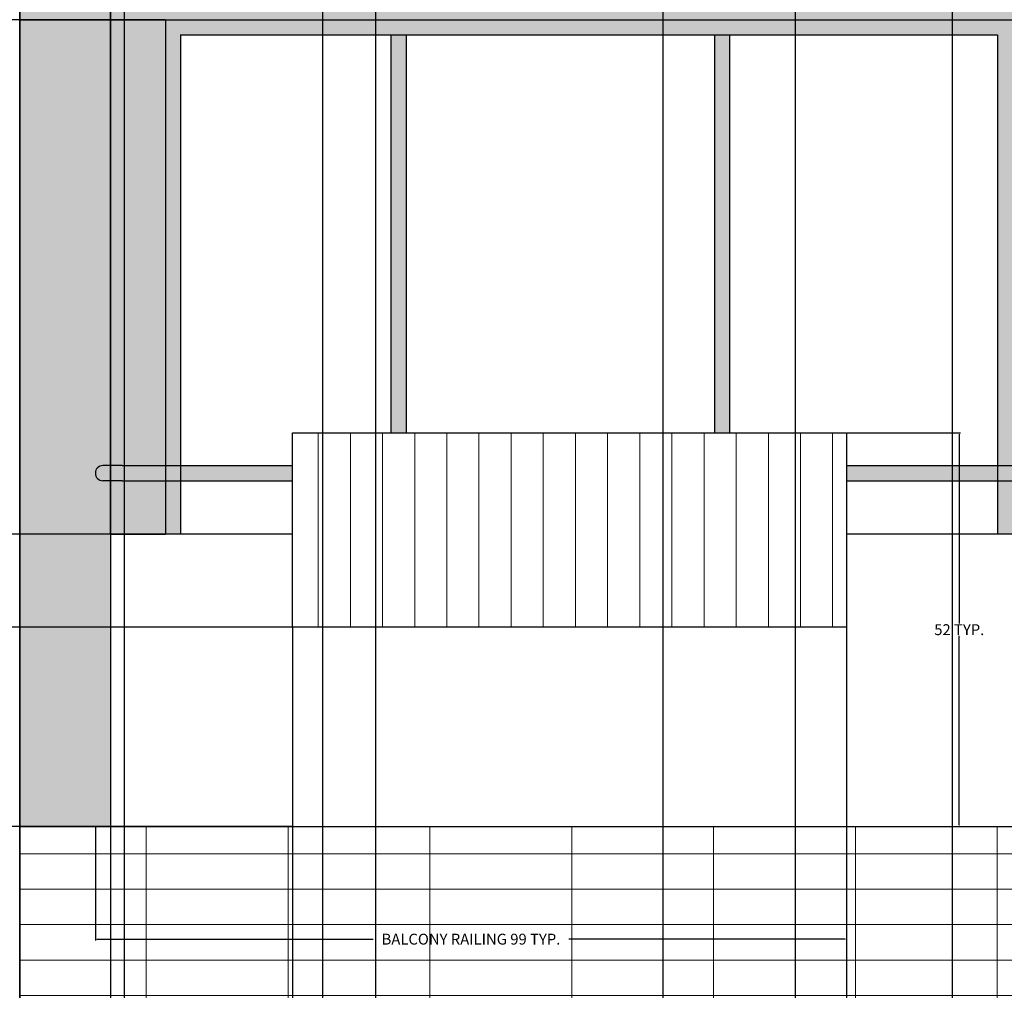
# Model space of a CAD drawing. Units: inches. Extents: x 241 to 943, y 109 to 1396.
# Tile 11 of 34: x 377 to 507, y 713 to 842. Entities that reach past the tile are written whole.
import ezdxf

# ---------------------------------------------------------------- set-up
doc = ezdxf.new("R2010")
doc.units = ezdxf.units.IN
doc.header["$MEASUREMENT"] = 0
for name, color, linetype, lineweight in [('A-ANNO-DIMS', 2, 'Continuous', 18), ('A-ELEV', 7, 'Continuous', 25), ('A-ELEV-SHAD', 9, 'Continuous', 13), ('A-GLAZ-PATT', 18, 'Continuous', 13), ('A-WALL-PATT', 8, 'Continuous', 13)]:
    doc.layers.add(name, color=color, linetype=linetype, lineweight=lineweight)
doc.styles.get("Standard").update_dxf_attribs({"font": 'arial.ttf'})
doc.dimstyles.get("Standard").update_dxf_attribs({"dimtxt": 1.4375, "dimasz": 0.18, "dimexe": 0.18, "dimexo": 0.0625, "dimgap": 0.09, "dimtad": 0, "dimtih": 1, "dimtoh": 1, "dimdec": 4, "dimzin": 0, "dimdsep": 46, "dimlunit": 4, "dimtxsty": 'Standard', "dimcen": 0.09, "dimadec": 0, "dimazin": 0, "dimtfac": 1, "dimtdec": 4, "dimtofl": 0, "dimtmove": 0, "dimatfit": 3, "dimfxl": 1, "dimtolj": 1, "dimtzin": 0, "dimarcsym": 0})

# ---------------------------------------------------------------- blocks, each defined once
blk = doc.blocks.new('BALCONY-RAIL')
for p, q in [((26.08, 26.37), (26.08, 52.06)), ((26.08, 52.06), (99.3, 52.06)), ((99.3, 52.06), (99.3, 26.37)), ((3.52, 47.73), (1, 47.73)), ((3.52, 47.73), (26.08, 47.73)), ((3.52, 45.73), (1, 45.73)), ((3.52, 45.73), (26.08, 45.73)), ((99.3, 26.37), (26.08, 26.37)), ((26.08, 26.37), (26.08, 0)), ((99.3, 26.37), (99.3, 0))]:
    blk.add_line(p, q)
blk.add_arc((1, 46.73), 1, 90, 270)
blk = doc.blocks.new('*D2')
at = {"layer": 'A-ANNO-DIMS', "color": 0, "lineweight": -2, "transparency": 16777216}
for p, q in [((387.04, 734.79), (387.04, 719.78)), ((486.34, 734.79), (486.34, 719.78)), ((387.22, 719.96), (423.76, 719.96)), ((486.16, 719.96), (449.62, 719.96))]:
    blk.add_line(p, q, dxfattribs=at)
at = {"layer": 'A-ANNO-DIMS', "color": 0, "transparency": 16777216}
for points in [[(387.22, 719.99), (387.22, 719.93), (387.04, 719.96)], [(486.16, 719.99), (486.16, 719.93), (486.34, 719.96)]]:
    blk.add_solid(points, dxfattribs=at)
at = {"layer": 'Defpoints', "color": 0, "transparency": 16777216}
for p in [(387.04, 734.85), (486.34, 734.85), (486.34, 719.96)]:
    blk.add_point(p, dxfattribs=at)
at = {"layer": 'A-ANNO-DIMS', "color": 0, "transparency": 16777216, "insert": (436.69, 719.96), "char_height": 1.4375, "attachment_point": 5}
blk.add_mtext('\\A1;BALCONY RAILING 99 TYP.', dxfattribs=at)
blk = doc.blocks.new('*D3')
at = {"layer": 'A-ANNO-DIMS', "color": 0, "lineweight": -2, "transparency": 16777216}
for p, q in [((486.4, 786.92), (501.42, 786.92)), ((501.24, 786.74), (501.24, 761.71)), ((501.24, 735.03), (501.24, 760.06)), ((486.4, 734.85), (501.42, 734.85))]:
    blk.add_line(p, q, dxfattribs=at)
at = {"layer": 'A-ANNO-DIMS', "color": 0, "transparency": 16777216}
for points in [[(501.21, 786.74), (501.27, 786.74), (501.24, 786.92)], [(501.21, 735.03), (501.27, 735.03), (501.24, 734.85)]]:
    blk.add_solid(points, dxfattribs=at)
at = {"layer": 'Defpoints', "color": 0, "transparency": 16777216}
for p in [(486.34, 786.92), (501.24, 786.92), (486.34, 734.85)]:
    blk.add_point(p, dxfattribs=at)
at = {"layer": 'A-ANNO-DIMS', "color": 0, "transparency": 16777216, "insert": (501.24, 760.88), "char_height": 1.4375, "attachment_point": 5}
blk.add_mtext('\\A1;52 TYP.', dxfattribs=at)
blk = doc.blocks.new('*D7')
at = {"layer": 'A-ANNO-DIMS', "color": 0, "lineweight": -2, "transparency": 16777216}
for p, q in [((508.24, 1336.12), (244.31, 1336.12)), ((244.49, 1335.94), (244.49, 753.25)), ((244.49, 168.92), (244.49, 751.6)), ((303.17, 168.74), (244.31, 168.74))]:
    blk.add_line(p, q, dxfattribs=at)
at = {"layer": 'A-ANNO-DIMS', "color": 0, "transparency": 16777216}
for points in [[(244.46, 1335.94), (244.52, 1335.94), (244.49, 1336.12)], [(244.46, 168.92), (244.52, 168.92), (244.49, 168.74)]]:
    blk.add_solid(points, dxfattribs=at)
at = {"layer": 'Defpoints', "color": 0, "transparency": 16777216}
for p in [(244.49, 1336.12), (508.31, 1336.12), (303.24, 168.74)]:
    blk.add_point(p, dxfattribs=at)
at = {"layer": 'A-ANNO-DIMS', "color": 0, "transparency": 16777216, "insert": (244.49, 752.43), "char_height": 1.438, "attachment_point": 5}
blk.add_mtext('\\A1;1167.4', dxfattribs=at)
blk = doc.blocks.new('*D8')
at = {"layer": 'A-ANNO-DIMS', "color": 0, "lineweight": -2, "transparency": 16777216}
for p, q in [((377.04, 396.94), (377.04, 1395.05)), ((377.22, 1394.87), (380.96, 1394.87)), ((390.71, 1394.87), (386.97, 1394.87)), ((390.89, 384.24), (390.89, 1395.05))]:
    blk.add_line(p, q, dxfattribs=at)
at = {"layer": 'A-ANNO-DIMS', "color": 0, "transparency": 16777216}
for points in [[(377.22, 1394.9), (377.22, 1394.84), (377.04, 1394.87)], [(390.71, 1394.9), (390.71, 1394.84), (390.89, 1394.87)]]:
    blk.add_solid(points, dxfattribs=at)
at = {"layer": 'Defpoints', "color": 0, "transparency": 16777216}
for p in [(390.89, 1394.87), (377.04, 396.88), (390.89, 384.18)]:
    blk.add_point(p, dxfattribs=at)
at = {"layer": 'A-ANNO-DIMS', "color": 0, "transparency": 16777216, "insert": (383.97, 1394.87), "char_height": 1.438, "attachment_point": 5}
blk.add_mtext('\\A1;13.856', dxfattribs=at)
blk = doc.blocks.new('*D9')
at = {"layer": 'A-ANNO-DIMS', "color": 0, "lineweight": -2, "transparency": 16777216}
for p, q in [((390.89, 384.24), (390.89, 1395.05)), ((391.07, 1394.87), (424.13, 1394.87)), ((461.93, 1394.87), (428.87, 1394.87)), ((462.11, 384.24), (462.11, 1395.05))]:
    blk.add_line(p, q, dxfattribs=at)
at = {"layer": 'A-ANNO-DIMS', "color": 0, "transparency": 16777216}
for points in [[(391.07, 1394.9), (391.07, 1394.84), (390.89, 1394.87)], [(461.93, 1394.9), (461.93, 1394.84), (462.11, 1394.87)]]:
    blk.add_solid(points, dxfattribs=at)
at = {"layer": 'Defpoints', "color": 0, "transparency": 16777216}
for p in [(462.11, 1394.87), (390.89, 384.18), (462.11, 384.18)]:
    blk.add_point(p, dxfattribs=at)
at = {"layer": 'A-ANNO-DIMS', "color": 0, "transparency": 16777216, "insert": (426.5, 1394.87), "char_height": 1.438, "attachment_point": 5}
blk.add_mtext('\\A1;71.21', dxfattribs=at)
blk = doc.blocks.new('*D10')
at = {"layer": 'A-ANNO-DIMS', "color": 0, "lineweight": -2, "transparency": 16777216}
for p, q in [((462.11, 384.24), (462.11, 1395.05)), ((462.29, 1394.87), (468.4, 1394.87)), ((479.42, 1394.87), (473.3, 1394.87)), ((479.6, 384.24), (479.6, 1395.05))]:
    blk.add_line(p, q, dxfattribs=at)
at = {"layer": 'A-ANNO-DIMS', "color": 0, "transparency": 16777216}
for points in [[(462.29, 1394.9), (462.29, 1394.84), (462.11, 1394.87)], [(479.42, 1394.9), (479.42, 1394.84), (479.6, 1394.87)]]:
    blk.add_solid(points, dxfattribs=at)
at = {"layer": 'Defpoints', "color": 0, "transparency": 16777216}
for p in [(479.6, 1394.87), (462.11, 384.18), (479.6, 384.18)]:
    blk.add_point(p, dxfattribs=at)
at = {"layer": 'A-ANNO-DIMS', "color": 0, "transparency": 16777216, "insert": (470.85, 1394.87), "char_height": 1.438, "attachment_point": 5}
blk.add_mtext('\\A1;17.49', dxfattribs=at)
blk = doc.blocks.new('*D11')
at = {"layer": 'A-ANNO-DIMS', "color": 0, "lineweight": -2, "transparency": 16777216}
for p, q in [((500.33, 384.24), (500.33, 1395.05)), ((500.51, 1394.87), (513.31, 1394.87)), ((530.05, 1394.87), (517.25, 1394.87)), ((530.23, 384.24), (530.23, 1395.05))]:
    blk.add_line(p, q, dxfattribs=at)
at = {"layer": 'A-ANNO-DIMS', "color": 0, "transparency": 16777216}
for points in [[(500.51, 1394.9), (500.51, 1394.84), (500.33, 1394.87)], [(530.05, 1394.9), (530.05, 1394.84), (530.23, 1394.87)]]:
    blk.add_solid(points, dxfattribs=at)
at = {"layer": 'Defpoints', "color": 0, "transparency": 16777216}
for p in [(530.23, 1394.87), (500.33, 384.18), (530.23, 384.18)]:
    blk.add_point(p, dxfattribs=at)
at = {"layer": 'A-ANNO-DIMS', "color": 0, "transparency": 16777216, "insert": (515.28, 1394.87), "char_height": 1.438, "attachment_point": 5}
blk.add_mtext('\\A1;29.9', dxfattribs=at)
blk = doc.blocks.new('*D35')
at = {"layer": 'A-ANNO-DIMS', "color": 0, "lineweight": -2, "transparency": 16777216}
for p, q in [((388.98, 773.49), (244.31, 773.49)), ((244.49, 773.31), (244.49, 755)), ((244.49, 735.03), (244.49, 753.35)), ((388.98, 734.85), (244.31, 734.85))]:
    blk.add_line(p, q, dxfattribs=at)
at = {"layer": 'A-ANNO-DIMS', "color": 0, "transparency": 16777216}
for points in [[(244.46, 773.31), (244.52, 773.31), (244.49, 773.49)], [(244.46, 735.03), (244.52, 735.03), (244.49, 734.85)]]:
    blk.add_solid(points, dxfattribs=at)
at = {"layer": 'Defpoints', "color": 0, "transparency": 16777216}
for p in [(244.49, 773.49), (389.04, 773.49), (389.04, 734.85)]:
    blk.add_point(p, dxfattribs=at)
at = {"layer": 'A-ANNO-DIMS', "color": 0, "transparency": 16777216, "insert": (244.49, 754.17), "char_height": 1.438, "attachment_point": 5}
blk.add_mtext('\\A1;38.64', dxfattribs=at)
blk = doc.blocks.new('*D36')
at = {"layer": 'A-ANNO-DIMS', "color": 0, "lineweight": -2, "transparency": 16777216}
for p, q in [((396.25, 841.54), (244.31, 841.54)), ((244.49, 841.36), (244.49, 808.34)), ((244.49, 773.67), (244.49, 806.69)), ((396.25, 773.49), (244.31, 773.49))]:
    blk.add_line(p, q, dxfattribs=at)
at = {"layer": 'A-ANNO-DIMS', "color": 0, "transparency": 16777216}
for points in [[(244.46, 841.36), (244.52, 841.36), (244.49, 841.54)], [(244.46, 773.67), (244.52, 773.67), (244.49, 773.49)]]:
    blk.add_solid(points, dxfattribs=at)
at = {"layer": 'Defpoints', "color": 0, "transparency": 16777216}
for p in [(244.49, 841.54), (396.31, 841.54), (396.31, 773.49)]:
    blk.add_point(p, dxfattribs=at)
at = {"layer": 'A-ANNO-DIMS', "color": 0, "transparency": 16777216, "insert": (244.49, 807.51), "char_height": 1.438, "attachment_point": 5}
blk.add_mtext('\\A1;68.05', dxfattribs=at)
blk = doc.blocks.new('*D61')
at = {"layer": 'A-ANNO-DIMS', "color": 0, "lineweight": -2, "transparency": 16777216}
for p, q in [((377.04, 400.89), (377.04, 1395.05)), ((377.22, 1394.87), (398.03, 1394.87)), ((423.93, 1394.87), (403.12, 1394.87)), ((424.11, 568.89), (424.11, 1395.05))]:
    blk.add_line(p, q, dxfattribs=at)
at = {"layer": 'A-ANNO-DIMS', "color": 0, "transparency": 16777216}
for points in [[(377.22, 1394.9), (377.22, 1394.84), (377.04, 1394.87)], [(423.93, 1394.9), (423.93, 1394.84), (424.11, 1394.87)]]:
    blk.add_solid(points, dxfattribs=at)
at = {"layer": 'Defpoints', "color": 0, "transparency": 16777216}
for p in [(424.11, 1394.87), (424.11, 568.83), (377.04, 400.83)]:
    blk.add_point(p, dxfattribs=at)
at = {"layer": 'A-ANNO-DIMS', "color": 0, "transparency": 16777216, "insert": (400.57, 1394.87), "char_height": 1.438, "attachment_point": 5}
blk.add_mtext('\\A1;47.07', dxfattribs=at)
blk = doc.blocks.new('*D62')
at = {"layer": 'A-ANNO-DIMS', "color": 0, "lineweight": -2, "transparency": 16777216}
for p, q in [((424.11, 568.89), (424.11, 1395.05)), ((424.29, 1394.87), (492.35, 1394.87)), ((565.02, 1394.87), (496.96, 1394.87)), ((565.2, 568.89), (565.2, 1395.05))]:
    blk.add_line(p, q, dxfattribs=at)
at = {"layer": 'A-ANNO-DIMS', "color": 0, "transparency": 16777216}
for points in [[(424.29, 1394.9), (424.29, 1394.84), (424.11, 1394.87)], [(565.02, 1394.9), (565.02, 1394.84), (565.2, 1394.87)]]:
    blk.add_solid(points, dxfattribs=at)
at = {"layer": 'Defpoints', "color": 0, "transparency": 16777216}
for p in [(565.2, 1394.87), (424.11, 568.83), (565.2, 568.83)]:
    blk.add_point(p, dxfattribs=at)
at = {"layer": 'A-ANNO-DIMS', "color": 0, "transparency": 16777216, "insert": (494.66, 1394.87), "char_height": 1.438, "attachment_point": 5}
blk.add_mtext('\\A1;141.1', dxfattribs=at)
blk = doc.blocks.new('*D65')
at = {"layer": 'A-ANNO-DIMS', "color": 0, "lineweight": -2, "transparency": 16777216}
for p, q in [((424.11, 700.85), (424.11, 1395.05)), ((424.29, 1394.87), (505.52, 1394.87)), ((592.77, 1394.87), (511.54, 1394.87)), ((592.95, 700.85), (592.95, 1395.05))]:
    blk.add_line(p, q, dxfattribs=at)
at = {"layer": 'A-ANNO-DIMS', "color": 0, "transparency": 16777216}
for points in [[(424.29, 1394.9), (424.29, 1394.84), (424.11, 1394.87)], [(592.77, 1394.9), (592.77, 1394.84), (592.95, 1394.87)]]:
    blk.add_solid(points, dxfattribs=at)
at = {"layer": 'Defpoints', "color": 0, "transparency": 16777216}
for p in [(592.95, 1394.87), (424.11, 700.79), (592.95, 700.79)]:
    blk.add_point(p, dxfattribs=at)
at = {"layer": 'A-ANNO-DIMS', "color": 0, "transparency": 16777216, "insert": (508.53, 1394.87), "char_height": 1.438, "attachment_point": 5}
blk.add_mtext('\\A1;168.85', dxfattribs=at)
blk = doc.blocks.new('*D67')
at = {"layer": 'A-ANNO-DIMS', "color": 0, "lineweight": -2, "transparency": 16777216}
for p, q in [((389.04, 773.55), (389.04, 1395.05)), ((389.22, 1394.87), (495.34, 1394.87)), ((607.64, 1394.87), (501.52, 1394.87)), ((607.82, 773.55), (607.82, 1395.05))]:
    blk.add_line(p, q, dxfattribs=at)
at = {"layer": 'A-ANNO-DIMS', "color": 0, "transparency": 16777216}
for points in [[(389.22, 1394.9), (389.22, 1394.84), (389.04, 1394.87)], [(607.64, 1394.9), (607.64, 1394.84), (607.82, 1394.87)]]:
    blk.add_solid(points, dxfattribs=at)
at = {"layer": 'Defpoints', "color": 0, "transparency": 16777216}
for p in [(607.82, 1394.87), (389.04, 773.49), (607.82, 773.49)]:
    blk.add_point(p, dxfattribs=at)
at = {"layer": 'A-ANNO-DIMS', "color": 0, "transparency": 16777216, "insert": (498.43, 1394.87), "char_height": 1.438, "attachment_point": 5}
blk.add_mtext('\\A1;218.77', dxfattribs=at)
blk = doc.blocks.new('*D79')
at = {"layer": 'A-ANNO-DIMS', "color": 0, "lineweight": -2, "transparency": 16777216}
for p, q in [((479.6, 384.24), (479.6, 1395.05)), ((479.78, 1394.87), (486.88, 1394.87)), ((500.15, 1394.87), (493.05, 1394.87)), ((500.33, 384.24), (500.33, 1395.05))]:
    blk.add_line(p, q, dxfattribs=at)
at = {"layer": 'A-ANNO-DIMS', "color": 0, "transparency": 16777216}
for points in [[(479.78, 1394.9), (479.78, 1394.84), (479.6, 1394.87)], [(500.15, 1394.9), (500.15, 1394.84), (500.33, 1394.87)]]:
    blk.add_solid(points, dxfattribs=at)
at = {"layer": 'Defpoints', "color": 0, "transparency": 16777216}
for p in [(500.33, 1394.87), (479.6, 384.18), (500.33, 384.18)]:
    blk.add_point(p, dxfattribs=at)
at = {"layer": 'A-ANNO-DIMS', "color": 0, "transparency": 16777216, "insert": (489.96, 1394.87), "char_height": 1.438, "attachment_point": 5}
blk.add_mtext('\\A1;20.736', dxfattribs=at)
blk = doc.blocks.new('*D91')
at = {"layer": 'A-ANNO-DIMS', "color": 0, "lineweight": -2, "transparency": 16777216}
for p, q in [((377.04, 1070.79), (377.04, 109.81)), ((389.04, 1070.79), (389.04, 109.81)), ((377.22, 109.99), (380.04, 109.99)), ((388.86, 109.99), (386.04, 109.99))]:
    blk.add_line(p, q, dxfattribs=at)
at = {"layer": 'A-ANNO-DIMS', "color": 0, "transparency": 16777216}
for points in [[(377.22, 110.02), (377.22, 109.96), (377.04, 109.99)], [(388.86, 110.02), (388.86, 109.96), (389.04, 109.99)]]:
    blk.add_solid(points, dxfattribs=at)
at = {"layer": 'Defpoints', "color": 0, "transparency": 16777216}
for p in [(377.04, 1070.85), (389.04, 1070.85), (389.04, 109.99)]:
    blk.add_point(p, dxfattribs=at)
at = {"layer": 'A-ANNO-DIMS', "color": 0, "transparency": 16777216, "insert": (383.04, 109.99), "char_height": 1.438, "attachment_point": 5}
blk.add_mtext('\\A1;12.004', dxfattribs=at)
blk = doc.blocks.new('*D99')
at = {"layer": 'A-ANNO-DIMS', "color": 0, "lineweight": -2, "transparency": 16777216}
for p, q in [((417.09, 181.71), (417.09, 1395.05)), ((417.27, 1394.87), (539.16, 1394.87)), ((667.21, 1394.87), (545.33, 1394.87)), ((667.39, 214.58), (667.39, 1395.05))]:
    blk.add_line(p, q, dxfattribs=at)
at = {"layer": 'A-ANNO-DIMS', "color": 0, "transparency": 16777216}
for points in [[(417.27, 1394.9), (417.27, 1394.84), (417.09, 1394.87)], [(667.21, 1394.9), (667.21, 1394.84), (667.39, 1394.87)]]:
    blk.add_solid(points, dxfattribs=at)
at = {"layer": 'Defpoints', "color": 0, "transparency": 16777216}
for p in [(667.39, 1394.87), (667.39, 214.52), (417.09, 181.65)]:
    blk.add_point(p, dxfattribs=at)
at = {"layer": 'A-ANNO-DIMS', "color": 0, "transparency": 16777216, "insert": (542.24, 1394.87), "char_height": 1.438, "attachment_point": 5}
blk.add_mtext('\\A1;250.30', dxfattribs=at)
blk = doc.blocks.new('*D147')
at = {"layer": 'A-ANNO-DIMS', "color": 0, "lineweight": -2, "transparency": 16777216}
for p, q in [((389.04, 734.79), (389.04, 109.81)), ((413.12, 734.79), (413.12, 109.81)), ((389.22, 109.99), (398, 109.99)), ((412.94, 109.99), (404.17, 109.99))]:
    blk.add_line(p, q, dxfattribs=at)
at = {"layer": 'A-ANNO-DIMS', "color": 0, "transparency": 16777216}
for points in [[(389.22, 110.02), (389.22, 109.96), (389.04, 109.99)], [(412.94, 110.02), (412.94, 109.96), (413.12, 109.99)]]:
    blk.add_solid(points, dxfattribs=at)
at = {"layer": 'Defpoints', "color": 0, "transparency": 16777216}
for p in [(389.04, 734.85), (413.12, 734.85), (413.12, 109.99)]:
    blk.add_point(p, dxfattribs=at)
at = {"layer": 'A-ANNO-DIMS', "color": 0, "transparency": 16777216, "insert": (401.08, 109.99), "char_height": 1.438, "attachment_point": 5}
blk.add_mtext('\\A1;24.076', dxfattribs=at)
blk = doc.blocks.new('*D148')
at = {"layer": 'A-ANNO-DIMS', "color": 0, "lineweight": -2, "transparency": 16777216}
for p, q in [((413.12, 734.79), (413.12, 109.81)), ((486.34, 734.79), (486.34, 109.81)), ((413.3, 109.99), (447.23, 109.99)), ((486.16, 109.99), (452.23, 109.99))]:
    blk.add_line(p, q, dxfattribs=at)
at = {"layer": 'A-ANNO-DIMS', "color": 0, "transparency": 16777216}
for points in [[(413.3, 110.02), (413.3, 109.96), (413.12, 109.99)], [(486.16, 110.02), (486.16, 109.96), (486.34, 109.99)]]:
    blk.add_solid(points, dxfattribs=at)
at = {"layer": 'Defpoints', "color": 0, "transparency": 16777216}
for p in [(413.12, 734.85), (486.34, 734.85), (486.34, 109.99)]:
    blk.add_point(p, dxfattribs=at)
at = {"layer": 'A-ANNO-DIMS', "color": 0, "transparency": 16777216, "insert": (449.73, 109.99), "char_height": 1.438, "attachment_point": 5}
blk.add_mtext('\\A1;73.22', dxfattribs=at)
blk = doc.blocks.new('*D149')
at = {"layer": 'A-ANNO-DIMS', "color": 0, "lineweight": -2, "transparency": 16777216}
for p, q in [((413.06, 761.23), (244.31, 761.23)), ((244.49, 761.05), (244.49, 748.87)), ((244.49, 735.03), (244.49, 747.22)), ((413.06, 734.85), (244.31, 734.85))]:
    blk.add_line(p, q, dxfattribs=at)
at = {"layer": 'A-ANNO-DIMS', "color": 0, "transparency": 16777216}
for points in [[(244.46, 761.05), (244.52, 761.05), (244.49, 761.23)], [(244.46, 735.03), (244.52, 735.03), (244.49, 734.85)]]:
    blk.add_solid(points, dxfattribs=at)
at = {"layer": 'Defpoints', "color": 0, "transparency": 16777216}
for p in [(244.49, 761.23), (413.12, 761.23), (413.12, 734.85)]:
    blk.add_point(p, dxfattribs=at)
at = {"layer": 'A-ANNO-DIMS', "color": 0, "transparency": 16777216, "insert": (244.49, 748.04), "char_height": 1.438, "attachment_point": 5}
blk.add_mtext('\\A1;26.375', dxfattribs=at)

msp = doc.modelspace()

# ---------------------------------------------------------------- hatches: boundary and pattern name
at = {"layer": 'A-ELEV-SHAD'}
h = msp.add_hatch(color=256, dxfattribs=at)
h.dxf.hatch_style = 1
h.paths.add_polyline_path([(508.3064, 1070.8538), (377.0391, 1070.8538), (377.0391, 1009.5382), (508.3064, 1009.5382)])
h.paths.add_polyline_path([(508.3064, 1238.8538), (377.0391, 1238.8538), (377.0391, 1177.5382), (508.3064, 1177.5382)])
h.paths.add_polyline_path([(581.3632, 902.8538), (568.1348, 902.8538), (553.5166, 902.8538), (377.0391, 902.8538), (377.0391, 841.5382), (553.5166, 841.5382), (564.8076, 841.5382), (581.3632, 841.5382)])
h.paths.add_polyline_path([(820.8374, 1275.9142), (747.7579, 1275.9142), (747.7579, 1238.8538), (820.8374, 1238.8538)])
h.paths.add_polyline_path([(820.8374, 1238.8538), (747.7579, 1238.8538), (747.9341, 1223.0633), (820.8374, 1223.0633)])
h.paths.add_polyline_path([(396.3125, 841.5382), (377.0391, 841.5382), (377.0391, 734.8538), (389.0429, 734.8538), (389.0429, 735.188), (389.0429, 773.4916), (396.3125, 773.4916), (396.3125, 780.5808), (390.5597, 780.5808), (388.0428, 780.5808, -1), (388.0428, 782.5808), (390.5597, 782.5808), (396.3125, 782.5808)])
h = msp.add_hatch(color=256, dxfattribs=at)
h.dxf.hatch_style = 1
h.paths.add_polyline_path([(537.4269, 698.7912), (534.1778, 698.7912), (534.1778, 659.3434), (537.4269, 659.3434)])
h.paths.add_polyline_path([(508.0803, 698.7912), (450.9259, 698.7912), (450.9259, 659.3434), (452.9259, 659.3434), (452.9259, 696.7912), (506.0803, 696.7912), (506.0803, 659.3434), (508.0803, 659.3434)])
h.paths.add_polyline_path([(481.5031, 696.7912), (479.5031, 696.7912), (479.5031, 659.3434), (481.5031, 659.3434)], flags=17)
h.paths.add_polyline_path([(481.5031, 657.3434), (479.5031, 657.3434), (479.5031, 653.3371), (481.5031, 653.3371)], flags=17)
h.paths.add_polyline_path([(508.0803, 657.3434), (506.0803, 657.3434), (506.0803, 653.3371), (452.9259, 653.3371), (452.9259, 657.3434), (450.9259, 657.3434), (450.9259, 651.3371), (508.0803, 651.3371)])
h.paths.add_polyline_path([(428.1173, 839.5382), (426.1173, 839.5382), (426.1173, 786.9154), (428.1173, 786.9154)], flags=17)
h.paths.add_polyline_path([(470.8692, 839.5382), (468.8692, 839.5382), (468.8692, 786.9154), (470.8692, 786.9154)], flags=17)
h.paths.add_polyline_path([(508.3064, 841.5382), (396.3125, 841.5382), (396.3125, 782.5808), (398.3125, 782.5808), (398.3125, 839.5382), (506.3064, 839.5382), (506.3064, 782.5808), (508.3064, 782.5808)])
h.paths.add_polyline_path([(398.3125, 780.5808), (396.3125, 780.5808), (396.3125, 773.4916), (398.3125, 773.4916)])
h.paths.add_polyline_path([(508.3064, 780.5808), (506.3064, 780.5808), (506.3064, 773.4916), (508.3064, 773.4916)])
h.paths.add_polyline_path([(715.6236, 841.5382), (678.2674, 841.5382), (678.2674, 734.8538), (715.6236, 734.8538)])
h.paths.add_polyline_path([(680.2674, 839.5382), (682.4526, 839.5382), (713.6236, 839.5382), (713.6236, 736.9235), (690.2047, 736.9235), (680.2674, 736.9235)], flags=16)
h.paths.add_polyline_path([(792.691, 841.5382), (747.7579, 841.5382), (747.7579, 734.8538), (754.5373, 734.8538), (754.5373, 736.9235), (754.5373, 839.5382), (756.7224, 839.5382), (787.8934, 839.5382), (787.8934, 765.9585), (792.691, 765.9585)])
h.paths.add_polyline_path([(659.2925, 1009.5382), (657.2925, 1009.5382), (657.2925, 902.8538), (659.2925, 902.8538)])
h.paths.add_polyline_path([(751.5078, 976.6275), (712.5839, 976.6275), (712.5839, 974.6275), (751.5078, 974.6275)])
h.paths.add_polyline_path([(470.8692, 1007.5382), (468.8692, 1007.5382), (468.8692, 954.9154), (470.8692, 954.9154)], flags=17)
h.paths.add_polyline_path([(508.3064, 1009.5382), (396.3125, 1009.5382), (396.3125, 950.5808), (398.3125, 950.5808), (398.3125, 1007.5382), (506.3064, 1007.5382), (506.3064, 950.5808), (508.3064, 950.5808)])
h.paths.add_polyline_path([(428.1173, 1007.5382), (426.1173, 1007.5382), (426.1173, 954.9154), (428.1173, 954.9154)], flags=17)
h.paths.add_polyline_path([(398.3125, 948.5808), (396.3125, 948.5808), (396.3125, 941.4916), (398.3125, 941.4916)])
h.paths.add_polyline_path([(508.3064, 948.5808), (506.3064, 948.5808), (506.3064, 941.4916), (508.3064, 941.4916)])
h.paths.add_polyline_path([(428.1173, 1175.5382), (426.1173, 1175.5382), (426.1173, 1122.9154), (428.1173, 1122.9154)], flags=17)
h.paths.add_polyline_path([(508.3064, 1177.5382), (396.3125, 1177.5382), (396.3125, 1118.5808), (398.3125, 1118.5808), (398.3125, 1175.5382), (506.3064, 1175.5382), (506.3064, 1118.5808), (506.8039, 1118.5808, -1), (506.8039, 1116.5808), (506.3064, 1116.5808), (506.3064, 1109.4916), (508.3064, 1109.4916)])
h.paths.add_polyline_path([(470.8692, 1175.5382), (468.8692, 1175.5382), (468.8692, 1122.9154), (470.8692, 1122.9154)], flags=17)
h.paths.add_polyline_path([(398.3125, 1116.5808), (396.3125, 1116.5808), (396.3125, 1109.4916), (398.3125, 1109.4916)], flags=17)
h.paths.add_polyline_path([(724.819, 1177.7336), (533.952, 1177.7336), (533.952, 1108.1686), (724.819, 1108.1686)])
h.paths.add_polyline_path([(535.952, 1175.7336), (722.819, 1175.7336), (722.819, 1110.1686), (535.952, 1110.1686)], flags=0)
h.paths.add_polyline_path([(622.521, 1136.0739), (643.4534, 1136.0739), (643.4534, 1134.0739), (622.521, 1134.0739)], flags=0)
h.paths.add_polyline_path([(722.819, 1175.7336), (535.952, 1175.7336), (535.952, 1110.1686), (722.819, 1110.1686)], flags=16)
h.paths.add_polyline_path([(565.947, 1151.5772), (535.952, 1151.5772), (535.952, 1149.5772), (565.947, 1149.5772)], flags=0)
at = {"layer": 'A-GLAZ-PATT'}
h = msp.add_hatch(dxfattribs=at)
h.set_pattern_fill('ANSI31', color=256, scale=34, angle=45)
h.paths.add_polyline_path([(486.3418, 786.9154), (413.1187, 786.9154), (413.1187, 761.2284), (486.3418, 761.2284)])
h.paths.add_polyline_path([(486.3418, 954.9154), (413.1187, 954.9154), (413.1187, 929.2284), (486.3418, 929.2284)])
h.paths.add_polyline_path([(462.1074, 289.6933), (390.895, 289.6933), (390.895, 277.4626), (390.895, 274.3507), (462.1074, 274.3507), (462.1074, 277.4626)])
h.paths.add_polyline_path([(500.3323, 289.6933), (479.596, 289.6933), (479.596, 274.3507), (500.3323, 274.3507)])
h.paths.add_polyline_path([(450.9259, 566.8295), (426.1086, 566.8295), (426.1086, 498.4395), (446.4348, 498.4395), (446.4348, 519.3754), (450.9259, 519.3754), (450.9259, 525.3816), (445.5808, 525.3816, -1), (445.5808, 527.3816), (450.9259, 527.3816)])
h.paths.add_polyline_path([(563.2023, 508.9074), (534.1778, 508.9074), (508.1906, 508.9074), (508.1906, 498.4395), (563.2023, 498.4395)])
h.paths.add_polyline_path([(747.6328, 700.7912), (712.0171, 700.7912), (712.0171, 628.4013), (747.6328, 628.4013)])
h.paths.add_polyline_path([(446.4348, 643.7483), (426.1086, 643.7483), (426.1086, 630.4013), (446.4348, 630.4013)])
h.paths.add_polyline_path([(564.8076, 841.5382), (553.5166, 841.5382), (508.3064, 841.5382), (508.3064, 782.5808), (564.8076, 782.5808)])
h.paths.add_polyline_path([(564.8076, 780.5808), (508.3064, 780.5808), (508.3064, 773.4916), (564.8076, 773.4916)])
h.paths.add_polyline_path([(792.691, 762.5799), (759.6248, 762.5799), (759.6248, 736.9235), (759.6248, 734.8538), (792.691, 734.8538)])
h.paths.add_polyline_path([(564.8076, 1009.5382), (553.5166, 1009.5382), (508.3064, 1009.5382), (508.3064, 950.5808), (562.3033, 950.5808, -1), (562.3033, 948.5808), (508.3064, 948.5808), (508.3064, 941.4916), (564.8076, 941.4916)])
h.paths.add_polyline_path([(486.3418, 1122.9154), (413.1187, 1122.9154), (413.1187, 1097.2284), (486.3418, 1097.2284)])
h = msp.add_hatch(color=256, dxfattribs=at)
h.dxf.hatch_style = 1
h.paths.add_polyline_path([(396.3125, 1118.5808), (390.5597, 1118.5808), (388.0428, 1118.5808, 1), (388.0428, 1116.5808), (390.5597, 1116.5808), (396.3125, 1116.5808)])
h.paths.add_polyline_path([(398.3125, 1118.5808), (396.3125, 1118.5808), (396.3125, 1116.5808), (398.3125, 1116.5808)])
h.paths.add_polyline_path([(413.1187, 1118.5808), (398.3125, 1118.5808), (398.3125, 1116.5808), (413.1187, 1116.5808)])
h.paths.add_polyline_path([(506.3064, 1118.5808), (486.3418, 1118.5808), (486.3418, 1116.5808), (506.3064, 1116.5808)])
h.paths.add_polyline_path([(506.8039, 1118.5808), (506.3064, 1118.5808), (506.3064, 1116.5808), (506.8039, 1116.5808, 1)])
h.paths.add_polyline_path([(396.3125, 950.5808), (390.5597, 950.5808), (388.0428, 950.5808, 1), (388.0428, 948.5808), (390.5597, 948.5808), (396.3125, 948.5808)])
h.paths.add_polyline_path([(398.3125, 950.5808), (396.3125, 950.5808), (396.3125, 948.5808), (398.3125, 948.5808)])
h.paths.add_polyline_path([(413.1187, 950.5808), (398.3125, 950.5808), (398.3125, 948.5808), (413.1187, 948.5808)])
h.paths.add_polyline_path([(506.3064, 950.5808), (486.3418, 950.5808), (486.3418, 948.5808), (506.3064, 948.5808)])
h.paths.add_polyline_path([(508.3064, 950.5808), (506.3064, 950.5808), (506.3064, 948.5808), (508.3064, 948.5808)])
h.paths.add_polyline_path([(562.3033, 950.5808), (508.3064, 950.5808), (508.3064, 948.5808), (562.3033, 948.5808, 1)])
h.paths.add_polyline_path([(396.3125, 782.5808), (390.5597, 782.5808), (388.0428, 782.5808, 1), (388.0428, 780.5808), (390.5597, 780.5808), (396.3125, 780.5808)])
h.paths.add_polyline_path([(398.3125, 782.5808), (396.3125, 782.5808), (396.3125, 780.5808), (398.3125, 780.5808)])
h.paths.add_polyline_path([(413.1187, 782.5808), (398.3125, 782.5808), (398.3125, 780.5808), (413.1187, 780.5808)])
h.paths.add_polyline_path([(506.3064, 782.5808), (486.3418, 782.5808), (486.3418, 780.5808), (506.3064, 780.5808)])
h.paths.add_polyline_path([(508.3064, 782.5808), (506.3064, 782.5808), (506.3064, 780.5808), (508.3064, 780.5808)])
h.paths.add_polyline_path([(564.8076, 782.5808), (508.3064, 782.5808), (508.3064, 780.5808), (564.8076, 780.5808)])
h.paths.add_polyline_path([(605.9087, 782.5808), (564.8076, 782.5808), (564.8076, 780.5808), (605.9087, 780.5808, 1)])
h.paths.add_polyline_path([(450.9259, 659.3434), (445.5808, 659.3434, 1), (445.5808, 657.3434), (450.9259, 657.3434)])
h.paths.add_polyline_path([(452.9259, 659.3434), (450.9259, 659.3434), (450.9259, 657.3434), (452.9259, 657.3434)])
h.paths.add_polyline_path([(506.0803, 659.3434), (452.9259, 659.3434), (452.9259, 657.3434), (506.0803, 657.3434)])
h.paths.add_polyline_path([(508.0803, 659.3434), (506.0803, 659.3434), (506.0803, 657.3434), (508.0803, 657.3434)])
h.paths.add_polyline_path([(563.2023, 659.3434), (537.4269, 659.3434), (537.4269, 657.3434), (563.2023, 657.3434)])
h.paths.add_polyline_path([(590.8792, 659.3434), (563.9297, 659.3434), (563.9297, 657.3434), (590.8792, 657.3434)])
h.paths.add_polyline_path([(563.9297, 659.3434), (563.2023, 659.3434), (563.2023, 657.3434), (563.9297, 657.3434)])
h.paths.add_polyline_path([(537.4269, 659.3434), (534.1778, 659.3434), (534.1778, 657.3434), (537.4269, 657.3434)])
h.paths.add_polyline_path([(534.1778, 659.3434), (508.0803, 659.3434), (508.0803, 657.3434), (534.1778, 657.3434)])
h.paths.add_polyline_path([(450.9259, 527.3816), (445.5808, 527.3816, 1), (445.5808, 525.3816), (450.9259, 525.3816)])
h.paths.add_polyline_path([(452.9259, 527.3816), (450.9259, 527.3816), (450.9259, 525.3816), (452.9259, 525.3816)])
h.paths.add_polyline_path([(479.5031, 527.3816), (452.9259, 527.3816), (452.9259, 525.3816), (479.5031, 525.3816)])
h.paths.add_polyline_path([(481.5031, 527.3816), (479.5031, 527.3816), (479.5031, 525.3816), (481.5031, 525.3816)])
h.paths.add_polyline_path([(506.0803, 527.3816), (481.5031, 527.3816), (481.5031, 525.3816), (506.0803, 525.3816)])
h.paths.add_polyline_path([(508.0803, 527.3816), (506.0803, 527.3816), (506.0803, 525.3816), (508.0803, 525.3816)])
h.paths.add_polyline_path([(563.2023, 527.3816), (508.0803, 527.3816), (508.0803, 525.3816), (563.2023, 525.3816)])
at = {"layer": 'A-WALL-PATT'}
h = msp.add_hatch(dxfattribs=at)
h.set_pattern_fill('GRATE', color=256, scale=150)
h.paths.add_polyline_path([(747.7579, 1238.8538), (747.7579, 1275.9142), (747.7579, 1336.1154), (508.3064, 1336.1154), (508.3064, 1275.9142), (508.3064, 1238.8538), (508.3064, 1177.5382), (508.3064, 1109.4916), (508.3064, 1070.8538), (553.5166, 1070.8538), (749.6328, 1070.8538)])
h.paths.add_polyline_path([(533.952, 1108.1686), (533.952, 1177.7336), (533.952, 1303.0286), (724.819, 1303.0286), (724.819, 1108.1686)], flags=16)
h.paths.add_polyline_path([(535.952, 1110.1686), (535.952, 1175.7336), (722.819, 1175.7336), (722.819, 1110.1686)], flags=0)
h.paths.add_polyline_path([(643.4534, 1134.0739), (622.521, 1134.0739), (622.521, 1136.0739), (643.4534, 1136.0739)], flags=0)
h.paths.add_polyline_path([(617.7594, 568.8295), (617.7594, 734.8538), (377.0391, 734.8538), (377.0391, 566.8538), (377.0391, 400.8295), (417.0913, 400.8295), (618.9643, 400.8295)])
h.paths.add_polyline_path([(424.1086, 496.4395), (424.1086, 568.8295), (565.2023, 568.8295), (565.2023, 496.4395)], flags=16)
h.paths.add_polyline_path([(426.1086, 498.4395), (426.1086, 566.8295), (563.2023, 566.8295), (563.2023, 508.9074), (563.2023, 498.4395)], flags=0)
h.paths.add_polyline_path([(508.0803, 508.9074), (508.0803, 519.3754), (450.9259, 519.3754), (450.9259, 525.3816), (445.5808, 525.3816, -1), (445.5808, 527.3816), (450.9259, 527.3816), (450.9259, 566.8295), (508.0803, 566.8295), (537.4269, 566.8295), (537.4269, 508.9074)], flags=0)
h.paths.add_polyline_path([(506.0803, 521.3754), (452.9259, 521.3754), (452.9259, 564.8295), (506.0803, 564.8295)], flags=0)
h.paths.add_polyline_path([(424.1086, 628.4013), (424.1086, 700.7912), (592.9542, 700.7912), (592.9542, 628.4013)], flags=16)
h.paths.add_polyline_path([(426.1086, 630.4013), (426.1086, 698.7912), (590.8792, 698.7912), (590.8792, 630.4013)], flags=0)
h.paths.add_polyline_path([(508.1906, 651.3371), (508.0803, 651.3371), (450.9259, 651.3371), (428.0291, 651.3371), (428.0291, 698.7912), (451.9767, 698.7912), (508.0803, 698.7912), (537.4269, 698.7912), (563.2023, 698.7912), (563.2023, 659.3434), (563.9297, 659.3434), (563.9297, 651.3371)], flags=0)
h.paths.add_polyline_path([(506.0803, 653.3371), (452.9259, 653.3371), (452.9259, 657.3434), (445.5808, 657.3434, -1), (445.5808, 659.3434), (452.9259, 659.3434), (452.9259, 696.7912), (506.0803, 696.7912)], flags=0)

# ---------------------------------------------------------------- linework, layer by layer
at = {"layer": 'A-ELEV'}
for p, q in [((377.0391, 734.8538), (377.0391, 902.8538)), ((377.0391, 841.5382), (553.5166, 841.5382)), ((396.3125, 841.5382), (396.3125, 773.4916)), ((398.3125, 839.5382), (398.3125, 773.4916)), ((398.3125, 839.5382), (506.3064, 839.5382)), ((426.1173, 839.5382), (426.1173, 786.9154)), ((428.1173, 839.5382), (428.1173, 786.9154)), ((468.8692, 839.5382), (468.8692, 786.9154)), ((470.8692, 839.5382), (470.8692, 786.9154)), ((506.3064, 839.5382), (506.3064, 773.4916)), ((486.3418, 782.5808), (605.9087, 782.5808)), ((486.3418, 780.5808), (605.9087, 780.5808)), ((389.0429, 773.4916), (389.0429, 735.188)), ((389.0429, 773.4916), (396.3125, 773.4916)), ((413.1187, 773.4916), (396.3125, 773.4916)), ((597.514, 773.4916), (486.3418, 773.4916)), ((377.0391, 566.8538), (377.0391, 734.8538)), ((377.0391, 734.8538), (792.691, 734.8538)), ((389.0429, 735.188), (389.0429, 734.8538))]:
    msp.add_line(p, q, dxfattribs=at)

# ---------------------------------------------------------------- block references
msp.add_blockref('BALCONY-RAIL', (387.043, 734.854), dxfattribs=at)

# ---------------------------------------------------------------- dimensions: what is measured, and where the dimension line sits
at = {"layer": 'A-ANNO-DIMS'}
for base, p1, p2, override, picture, middle in [((390.895, 1394.8654), (377.0391, 396.8782), (390.895, 384.1784), {"dimdec": 3, "dimlfac": 1, "dimrnd": 0, "dimzin": 0, "dimdsep": 46, "dimlunit": 2}, '*D8', (383.9671, 1394.8654)), ((424.1086, 1394.8654), (377.0391, 400.8295), (424.1086, 568.8295), {"dimdec": 2, "dimlfac": 1, "dimrnd": 0, "dimzin": 0, "dimdsep": 46, "dimlunit": 2}, '*D61', (400.5739, 1394.8654)), ((607.8162, 1394.8654), (389.0429, 773.4916), (607.8162, 773.4916), {"dimdec": 2, "dimlfac": 1, "dimrnd": 0, "dimzin": 0, "dimdsep": 46, "dimlunit": 2}, '*D67', (498.4295, 1394.8654)), ((462.1074, 1394.8654), (390.895, 384.1784), (462.1074, 384.1784), {"dimdec": 2, "dimlfac": 1, "dimrnd": 0, "dimzin": 0, "dimdsep": 46, "dimlunit": 2}, '*D9', (426.5012, 1394.8654)), ((667.3935, 1394.8654), (417.0913, 181.649), (667.3935, 214.5189), {"dimdec": 2, "dimlfac": 1, "dimrnd": 0, "dimzin": 0, "dimdsep": 46, "dimlunit": 2}, '*D99', (542.2424, 1394.8654)), ((565.2023, 1394.8654), (424.1086, 568.8295), (565.2023, 568.8295), {"dimdec": 1, "dimlfac": 1, "dimrnd": 0, "dimzin": 0, "dimdsep": 46, "dimlunit": 2}, '*D62', (494.6554, 1394.8654)), ((592.9542, 1394.8654), (424.1086, 700.7912), (592.9542, 700.7912), {"dimdec": 2, "dimlfac": 1, "dimrnd": 0, "dimzin": 0, "dimdsep": 46, "dimlunit": 2}, '*D65', (508.5314, 1394.8654)), ((479.596, 1394.8654), (462.1074, 384.1784), (479.596, 384.1784), {"dimdec": 2, "dimlfac": 1, "dimrnd": 0, "dimzin": 0, "dimdsep": 46, "dimlunit": 2}, '*D10', (470.8517, 1394.8654)), ((500.3323, 1394.8654), (479.596, 384.1784), (500.3323, 384.1784), {"dimdec": 3, "dimlfac": 1, "dimrnd": 0, "dimzin": 0, "dimdsep": 46, "dimlunit": 2}, '*D79', (489.9641, 1394.8654)), ((530.2303, 1394.8654), (500.3323, 384.1784), (530.2303, 384.1784), {"dimdec": 1, "dimlfac": 1, "dimrnd": 0, "dimzin": 0, "dimdsep": 46, "dimlunit": 2}, '*D11', (515.2813, 1394.8654)), ((389.0429, 109.9907), (377.0391, 1070.8538), (389.0429, 1070.8538), {"dimdec": 3, "dimlfac": 1, "dimrnd": 0, "dimzin": 0, "dimdsep": 46, "dimlunit": 2}, '*D91', (383.041, 109.9907)), ((413.1187, 109.9907), (389.0429, 734.8538), (413.1187, 734.8538), {"dimdec": 3, "dimlfac": 1, "dimrnd": 0, "dimzin": 0, "dimdsep": 46, "dimlunit": 2}, '*D147', (401.0808, 109.9907)), ((486.3418, 109.9907), (413.1187, 734.8538), (486.3418, 734.8538), {"dimdec": 2, "dimlfac": 1, "dimrnd": 0, "dimzin": 0, "dimdsep": 46, "dimlunit": 2}, '*D148', (449.7303, 109.9907))]:
    dim = msp.add_linear_dim(base=base, p1=p1, p2=p2, dimstyle='Standard', override=override, dxfattribs=at)
    dim.commit()
    dim.dimension.update_dxf_attribs({"geometry": picture, "text_midpoint": middle})
for base, p1, p2, override, picture, middle in [((244.4858, 1336.1154), (303.2358, 168.7407), (508.3064, 1336.1154), {"dimdec": 1, "dimlfac": 1, "dimrnd": 0, "dimzin": 0, "dimdsep": 46, "dimlunit": 2}, '*D7', (244.4858, 752.4281)), ((244.4858, 841.5382), (396.3125, 773.4916), (396.3125, 841.5382), {"dimdec": 2, "dimlfac": 1, "dimrnd": 0, "dimzin": 0, "dimdsep": 46, "dimlunit": 2}, '*D36', (244.4858, 807.5149)), ((244.4858, 773.4916), (389.0429, 734.8538), (389.0429, 773.4916), {"dimdec": 2, "dimlfac": 1, "dimrnd": 0, "dimzin": 0, "dimdsep": 46, "dimlunit": 2}, '*D35', (244.4858, 754.1727)), ((244.4858, 761.2284), (413.1187, 734.8538), (413.1187, 761.2284), {"dimdec": 3, "dimlfac": 1, "dimrnd": 0, "dimzin": 0, "dimdsep": 46, "dimlunit": 2}, '*D149', (244.4858, 748.0411))]:
    dim = msp.add_linear_dim(base=base, p1=p1, p2=p2, angle=90, dimstyle='Standard', override=override, dxfattribs=at)
    dim.commit()
    dim.dimension.update_dxf_attribs({"geometry": picture, "text_midpoint": middle})
dim = msp.add_linear_dim(base=(501.2367, 786.9154), p1=(486.3418, 734.8538), p2=(486.3418, 786.9154), angle=90, text='<> TYP.', dimstyle='Standard', override={"dimdec": 0, "dimrnd": 0, "dimzin": 0, "dimlunit": 2}, dxfattribs=at)
dim.commit()
dim.dimension.update_dxf_attribs({"geometry": '*D3', "text_midpoint": (501.2367, 760.8846)})
dim = msp.add_linear_dim(base=(486.3418, 719.959), p1=(387.0428, 734.8538), p2=(486.3418, 734.8538), text='BALCONY RAILING <> TYP.', dimstyle='Standard', override={"dimdec": 0, "dimrnd": 0, "dimzin": 0, "dimlunit": 2}, dxfattribs=at)
dim.commit()
dim.dimension.update_dxf_attribs({"geometry": '*D2', "text_midpoint": (436.6923, 719.959)})

doc.saveas('drawing.dxf')
